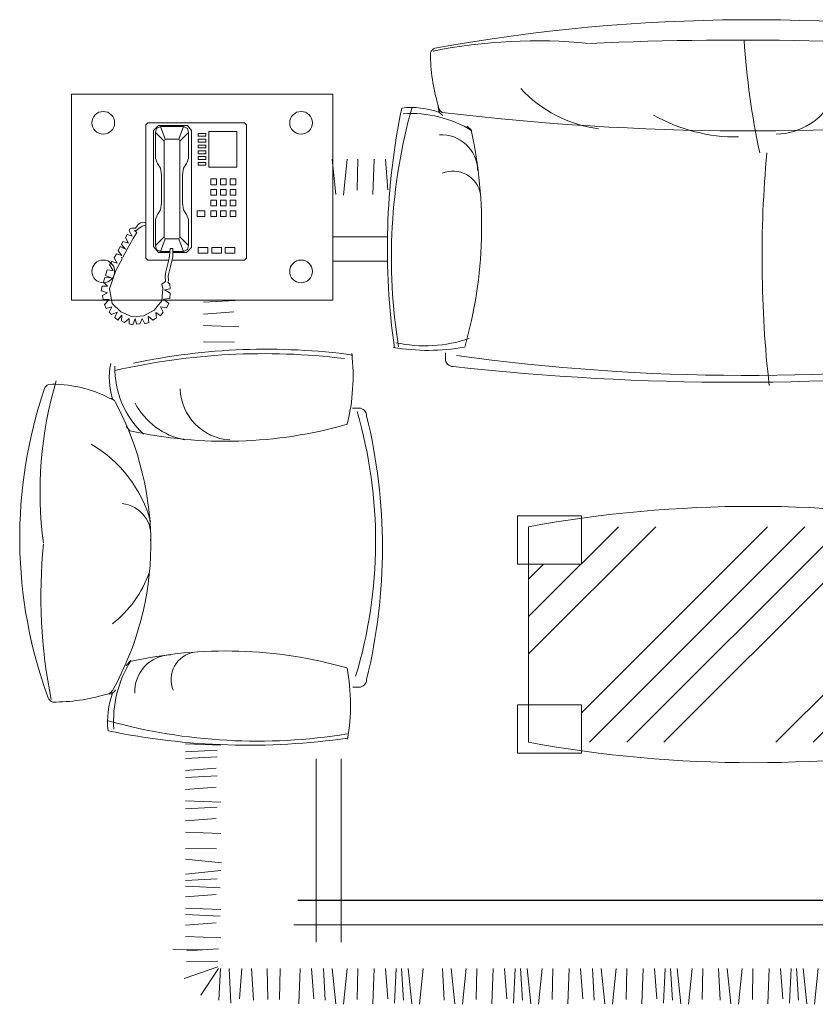
# Model space of a CAD drawing. Units: inches. Extents: x 1961 to 3038, y 800 to 1438.
# Tile 8 of 13: x 2866 to 2920, y 1028 to 1096. Entities that reach past the tile are written whole.
import ezdxf

# ---------------------------------------------------------------- set-up
doc = ezdxf.new("R2010")
doc.units = ezdxf.units.IN
doc.layers.add('A-FURN', color=8, linetype='Continuous', lineweight=18)

# ---------------------------------------------------------------- blocks, each defined once
blk = doc.blocks.new('A$C28C76B35')
for p, q in [((1695.2, 4127.1, -618.7), (2191.4, 4127.1, -618.7)), ((1695.2, 3498.2, -618.7), (1695.2, 4127.1, -618.7)), ((2191.4, 4127.1, -618.7), (2191.4, 3498.2, -618.7)), ((1713.2, 4040.6, -1415), (1717.4, 4055.2, -1415)), ((1717.2, 4055.4, 1292.3), (1729.2, 4053, 1292.3)), ((1660.8, 4030.7, -1415), (1666.5, 4036.8, -1415)), ((1666.5, 4017.5, -1415), (1660.8, 4030.7, -1415)), ((1666.5, 4036.8, -1415), (1679.2, 4030.2, -1415)), ((1675, 4043.9, -1415), (1684.4, 4047.6, -1415)), ((1679.2, 4030.2, -1415), (1675, 4043.9, -1415)), ((1684.4, 4047.6, -1415), (1697.1, 4036.3, -1415)), ((1722.6, 4035.9, -1415), (1687.2, 4029.3, -1415)), ((1696.5, 4050.9, 1292.3), (1706.1, 4052.8, 1292.3)), ((1697.1, 4036.3, -1415), (1696.7, 4050.9, -1415)), ((1706.1, 4052.8, -1415), (1713.2, 4040.6, -1415)), ((1766.9, 4020.3, -1415), (1722.6, 4035.9, -1415)), ((1729.2, 4052.8, -1415), (1729.2, 4040.1, -1415)), ((1729.2, 4040.1, -1415), (1738.6, 4050, -1415)), ((1738.4, 4050.1, 1292.3), (1749.4, 4046.8, 1292.3)), ((1749.5, 4046.7, -1415), (1749, 4031.6, -1415)), ((1749, 4031.6, -1415), (1754.2, 4045.3, -1415)), ((1754.2, 4045.3, -1415), (1768.3, 4041, -1415)), ((1768.3, 4041, -1415), (1766.9, 4026.9, -1415)), ((1766.9, 4026.9, -1415), (1780.6, 4035.4, -1415)), ((1780.6, 4035.4, -1415), (1788.2, 4030.2, -1415)), ((1788.2, 4030.2, -1415), (1784.4, 4017, -1415)), ((1641.5, 3999.6, -1415), (1645.3, 4007.1, -1415)), ((1645.3, 4007.1, -1415), (1659.4, 4005.7, -1415)), ((1647.2, 4015.6, -1415), (1653.8, 4023.1, -1415)), ((1659.4, 4005.7, -1415), (1647.2, 4015.6, -1415)), ((1653.8, 4023.1, -1415), (1666.5, 4017.5, -1415)), ((1667, 4008.5, -1415), (1655.2, 3981.2, -1415)), ((1687.2, 4029.3, -1415), (1667, 4008.5, -1415)), ((1794.3, 4005.2, -1415), (1766.9, 4020.3, -1415)), ((1784.4, 4017, -1415), (1797.1, 4024.1, -1415)), ((1798.1, 4006.6, -1415), (1794.3, 4005.2, -1415)), ((1797.1, 4024.1, -1415), (1807, 4018.9, -1415)), ((1799, 4003.3, -1415), (1798.1, 4006.6, -1415)), ((1807, 4018.9, -1415), (1802.8, 4006.2, -1415)), ((1802.8, 4006.2, -1415), (1813.6, 4014.7, -1415)), ((1813.6, 4014.7, -1415), (1824, 4009.9, -1415)), ((1824, 4009.9, -1415), (1818.3, 3997.2, -1415)), ((1818.3, 3997.2, -1415), (1829.2, 4007.1, -1415)), ((1829.2, 4007.1, -1415), (1836.7, 4003.3, -1415)), ((1635.8, 3979.3, -1415), (1638.2, 3988.3, -1415)), ((1638.2, 3988.3, -1415), (1650.9, 3988.7, -1415)), ((1650.9, 3988.7, -1415), (1641.5, 3999.6, -1415)), ((1818.3, 3993.5, -1415), (1799, 4003.3, -1415)), ((1843.8, 3978.4, -1415), (1818.3, 3993.5, -1415)), ((1836.7, 4003.3, -1415), (1832.5, 3989.7, -1415)), ((1832.5, 3989.7, -1415), (1846.2, 3997.2, -1415)), ((1846.2, 3997.2, -1415), (1853.2, 3993.5, -1415)), ((1853.2, 3993.5, -1415), (1849.5, 3981.2, -1415)), ((1849.5, 3981.2, -1415), (1861.7, 3988.7, -1415)), ((1861.7, 3988.7, -1415), (1866.9, 3986.9, -1415)), ((1866.9, 3986.9, -1415), (1868.3, 3981.7, -1415)), ((1650.9, 3974.1, -1415), (1635.8, 3979.3, -1415)), ((1637.3, 3970.8, -1415), (1650.9, 3974.1, -1415)), ((1638.2, 3962.8, -1415), (1637.3, 3970.8, -1415)), ((1650.9, 3957.2, -1415), (1638.2, 3962.8, -1415)), ((1655.2, 3981.2, -1415), (1657.5, 3952.9, -1415)), ((1857.9, 3969.9, -1415), (1843.8, 3978.4, -1415)), ((1862.7, 3975.5, -1415), (1857.9, 3969.9, -1415)), ((1862.7, 3970.8, -1415), (1862.7, 3975.5, -1415)), ((1865.5, 3968, -1415), (1862.7, 3970.8, -1415)), ((1869.7, 3961.9, -1415), (1865.5, 3968, -1415)), ((1868.3, 3981.7, -1415), (1868.8, 3973.2, -1415)), ((1868.8, 3973.2, -1415), (1877.7, 3966.6, -1415)), ((1873.5, 3956.7, -1415), (1869.7, 3961.9, -1415)), ((1877.7, 3966.6, -1415), (1881, 3960.9, -1415)), ((1881, 3960.9, -1415), (1882.4, 3948.1, -1415)), ((1638.2, 3951, -1415), (1650.9, 3957.2, -1415)), ((1641, 3941.1, -1415), (1638.2, 3951, -1415)), ((1656.6, 3942.6, -1415), (1641, 3941.1, -1415)), ((1647.2, 3931.2, -1415), (1656.6, 3942.6, -1415)), ((1657.5, 3952.9, -1415), (1670.7, 3927.9, -1415)), ((1796.3, 3948.1, -1415), (1791.6, 3943.4, -1415)), ((1791.6, 3943.4, -1415), (1791.6, 3893.2, -1415)), ((2117.6, 3948.1, -1415), (1796.3, 3948.1, -1415)), ((1875.4, 3948.1, -1415), (1873.5, 3956.7, -1415)), ((2122.3, 3943.4, -1415), (2117.6, 3948.1, -1415)), ((2122.3, 3710.5, -1415), (2122.3, 3943.4, -1415)), ((1652.8, 3922.3, -1415), (1647.2, 3931.2, -1415)), ((1665.6, 3924.2, -1415), (1652.8, 3922.3, -1415)), ((1657.5, 3913.3, -1415), (1665.6, 3924.2, -1415)), ((1666, 3906.3, -1415), (1657.5, 3913.3, -1415)), ((1679.2, 3912.9, -1415), (1666, 3906.3, -1415)), ((1670.7, 3927.9, -1415), (1693.4, 3910, -1415)), ((1676.4, 3898.7, -1415), (1679.2, 3912.9, -1415)), ((1824.2, 3929.4, -1415), (1810.2, 3917.8, -1415)), ((1810.2, 3917.8, -1415), (1810.2, 3890.5, -1415)), ((1812.6, 3913.1, -1415), (1817.2, 3922.4, -1415)), ((1812.6, 3890.3, -1415), (1812.6, 3913.1, -1415)), ((1842.8, 3901.5, -1415), (1812.6, 3913.1, -1415)), ((1817.2, 3922.4, -1415), (1826.5, 3924.8, -1415)), ((2103.6, 3929.4, -1415), (1824.2, 3929.4, -1415)), ((1826.5, 3924.8, -1415), (1889.4, 3924.8, -1415)), ((1826.5, 3924.8, -1415), (1847.5, 3903.8, -1415)), ((1889.4, 3924.8, -1415), (1901.1, 3920.1, -1415)), ((1901.1, 3920.1, -1415), (1912.7, 3913.1, -1415)), ((1912.7, 3913.1, -1415), (1929, 3910.8, -1415)), ((2012.8, 3913.1, -1415), (1996.5, 3910.8, -1415)), ((2024.5, 3920.1, -1415), (2012.8, 3913.1, -1415)), ((2036.1, 3924.8, -1415), (2024.5, 3920.1, -1415)), ((2099, 3924.8, -1415), (2036.1, 3924.8, -1415)), ((2099, 3924.8, -1415), (2078, 3903.8, -1415)), ((2082.7, 3901.5, -1415), (2112.9, 3913.1, -1415)), ((2108.3, 3922.4, -1415), (2099, 3924.8, -1415)), ((2115.3, 3917.8, -1415), (2103.6, 3929.4, -1415)), ((2112.9, 3913.1, -1415), (2108.3, 3922.4, -1415)), ((2112.9, 3857.2, -1415), (2112.9, 3913.1, -1415)), ((2115.3, 3847.9, -1415), (2115.3, 3917.8, -1415)), ((1687.2, 3892.6, -1415), (1676.4, 3898.7, -1415)), ((1697.6, 3905.8, -1415), (1687.2, 3892.6, -1415)), ((1693.4, 3910, -1415), (1723.1, 3907.7, -1415)), ((1699, 3890.7, -1415), (1697.6, 3905.8, -1415)), ((1711.8, 3889.8, -1415), (1699, 3890.7, -1415)), ((1719.8, 3903, -1415), (1711.8, 3889.8, -1415)), ((1722.1, 3889.3, -1415), (1719.8, 3903, -1415)), ((1733.5, 3890.2, -1415), (1722.1, 3889.3, -1415)), ((1723.1, 3907.7, -1415), (1733.9, 3909.6, -1415)), ((1738.6, 3895.4, -1415), (1733.5, 3890.2, -1415)), ((1733.9, 3909.6, -1415), (1740.1, 3901.1, -1415)), ((1741.5, 3894, -1415), (1738.6, 3895.4, -1415)), ((1740.1, 3901.1, -1415), (1752.3, 3901.6, -1415)), ((1753.7, 3894.5, -1415), (1741.5, 3894, -1415)), ((1752.3, 3901.6, -1415), (1763.6, 3900.1, -1415)), ((1775.9, 3888.8, -1415), (1753.7, 3894.5, -1415)), ((1763.6, 3900.1, -1415), (1785.8, 3894.5, -1415)), ((1799.5, 3883.2, -1415), (1775.9, 3888.8, -1415)), ((1785.8, 3894.5, -1415), (1800.9, 3891.2, -1415)), ((1800.9, 3891.2, -1415), (1819.6, 3889.8, -1415)), ((1819.6, 3889.8, -1415), (1819.6, 3882.9, -1415)), ((1847.5, 3903.8, -1415), (1842.8, 3901.5, -1415)), ((1842.8, 3901.5, -1415), (1842.8, 3868.9, -1415)), ((1973.2, 3903.8, -1415), (1847.5, 3903.8, -1415)), ((1929, 3910.8, -1415), (1973.2, 3910.8, -1415)), ((1996.5, 3910.8, -1415), (1973.2, 3910.8, -1415)), ((1973.2, 3903.8, -1415), (2078, 3903.8, -1415)), ((2078, 3903.8, -1415), (2082.7, 3901.5, -1415)), ((2082.7, 3901.5, -1415), (2082.7, 3868.9, -1415)), ((131, 3801, -715.1), (132.6, 3883.3, -715.1)), ((1791.6, 3885.1, -1415), (1791.6, 3710.5, -1415)), ((1819.6, 3882.9, -1415), (1799.5, 3883.2, -1415)), ((1810.2, 3883, -1415), (1810.2, 3850.3, -1415)), ((1812.6, 3857.2, -1415), (1812.6, 3883, -1415)), ((1842.8, 3868.9, -1415), (1812.6, 3857.2, -1415)), ((1826.5, 3845.6, -1415), (1847.5, 3866.6, -1415)), ((1847.5, 3866.6, -1415), (1842.8, 3868.9, -1415)), ((1973.2, 3866.6, -1415), (1847.5, 3866.6, -1415)), ((1973.2, 3866.6, -1415), (2078, 3866.6, -1415)), ((2078, 3866.6, -1415), (2082.7, 3868.9, -1415)), ((2099, 3845.6, -1415), (2078, 3866.6, -1415)), ((2082.7, 3868.9, -1415), (2112.9, 3857.2, -1415)), ((89.9, 3775.3, -715.1), (61.8, 3856, -715.1)), ((103.7, 3775.7, -715.1), (102.2, 3850.5, -715.1)), ((133.3, 3773.3, -715.1), (129, 3849.6, -715.1)), ((162.9, 3852.6, -715.1), (160, 3767.7, -715.1)), ((190.2, 3852.6, -715.1), (196, 3779.2, -715.1)), ((216.2, 3852.6, -715.1), (211.9, 3769.2, -715.1)), ((231.4, 3852.6, -715.1), (228.6, 3767.7, -715.1)), ((258.8, 3852.6, -715.1), (264.6, 3779.2, -715.1)), ((284.7, 3852.6, -715.1), (280.4, 3769.2, -715.1)), ((297.7, 3852.6, -715.1), (302, 3776.4, -715.1)), ((313.5, 3852.6, -715.1), (322.2, 3767.7, -715.1)), ((349.5, 3852.6, -715.1), (340.9, 3766.3, -715.1)), ((375.4, 3852.6, -715.1), (374, 3777.8, -715.1)), ((414.3, 3852.6, -715.1), (411.5, 3767.7, -715.1)), ((441.7, 3852.6, -715.1), (447.5, 3779.2, -715.1)), ((470.4, 3852.6, -715.1), (474.7, 3776.4, -715.1)), ((489.7, 3852.6, -715.1), (486.9, 3767.7, -715.1)), ((517.1, 3852.6, -715.1), (522.9, 3779.2, -715.1)), ((545.8, 3852.6, -715.1), (550.1, 3776.4, -715.1)), ((562.8, 3852.6, -715.1), (568.6, 3779.2, -715.1)), ((591.5, 3852.6, -715.1), (595.8, 3776.4, -715.1)), ((607.5, 3852.6, -715.1), (611.8, 3776.4, -715.1)), ((626.8, 3852.6, -715.1), (623.9, 3767.7, -715.1)), ((1810.2, 3850.3, -1415), (1821.9, 3838.6, -1415)), ((1812.6, 3857.2, -1415), (1817.2, 3847.9, -1415)), ((1817.2, 3847.9, -1415), (1826.5, 3845.6, -1415)), ((1826.5, 3845.6, -1415), (1889.4, 3845.6, -1415)), ((1889.4, 3845.6, -1415), (1901.1, 3850.3, -1415)), ((1901.1, 3850.3, -1415), (1912.7, 3857.2, -1415)), ((1912.7, 3857.2, -1415), (1929, 3859.6, -1415)), ((1929, 3859.6, -1415), (1973.2, 3859.6, -1415)), ((1996.5, 3859.6, -1415), (1973.2, 3859.6, -1415)), ((2012.8, 3857.2, -1415), (1996.5, 3859.6, -1415)), ((2024.5, 3850.3, -1415), (2012.8, 3857.2, -1415)), ((2036.1, 3845.6, -1415), (2024.5, 3850.3, -1415)), ((2099, 3845.6, -1415), (2036.1, 3845.6, -1415)), ((2108.3, 3847.9, -1415), (2099, 3845.6, -1415)), ((2103.6, 3838.6, -1415), (2115.3, 3847.9, -1415)), ((2112.9, 3857.2, -1415), (2108.3, 3847.9, -1415)), ((1807.9, 3822.3, -1415), (1821.9, 3822.3, -1415)), ((1807.9, 3799, -1415), (1807.9, 3822.3, -1415)), ((1821.9, 3838.6, -1415), (2103.6, 3838.6, -1415)), ((1821.9, 3822.3, -1415), (1821.9, 3799, -1415)), ((1910.4, 3824.6, -1415), (1896.4, 3824.6, -1415)), ((1896.4, 3824.6, -1415), (1896.4, 3806, -1415)), ((1910.4, 3806, -1415), (1910.4, 3824.6, -1415)), ((2019.8, 3822.3, -1415), (2026.8, 3822.3, -1415)), ((2019.8, 3803.7, -1415), (2019.8, 3822.3, -1415)), ((2026.8, 3822.3, -1415), (2026.8, 3803.7, -1415)), ((2033.8, 3822.3, -1415), (2040.8, 3822.3, -1415)), ((2033.8, 3803.7, -1415), (2033.8, 3822.3, -1415)), ((2040.8, 3822.3, -1415), (2040.8, 3803.7, -1415)), ((2047.7, 3822.3, -1415), (2054.7, 3822.3, -1415)), ((2047.7, 3803.7, -1415), (2047.7, 3822.3, -1415)), ((2054.7, 3822.3, -1415), (2054.7, 3803.7, -1415)), ((2061.7, 3822.3, -1415), (2068.7, 3822.3, -1415)), ((2061.7, 3803.7, -1415), (2061.7, 3822.3, -1415)), ((2068.7, 3822.3, -1415), (2068.7, 3803.7, -1415)), ((2075.7, 3822.3, -1415), (2082.7, 3822.3, -1415)), ((2075.7, 3803.7, -1415), (2075.7, 3822.3, -1415)), ((2082.7, 3822.3, -1415), (2082.7, 3803.7, -1415)), ((2089.7, 3822.3, -1415), (2096.6, 3822.3, -1415)), ((2089.7, 3803.7, -1415), (2089.7, 3822.3, -1415)), ((2096.6, 3822.3, -1415), (2096.6, 3803.7, -1415)), ((85.9, 3773.7, -715.1), (22.2, 3815.6, -715.1)), ((1595.1, 3809.5, -715.1), (1593.7, 3734.7, -715.1)), ((1634, 3809.5, -715.1), (1631.1, 3724.6, -715.1)), ((1661.4, 3809.5, -715.1), (1667.1, 3736.1, -715.1)), ((1690.1, 3809.5, -715.1), (1694.4, 3733.2, -715.1)), ((1821.9, 3799, -1415), (1807.9, 3799, -1415)), ((1896.4, 3806, -1415), (1910.4, 3806, -1415)), ((2101.3, 3796.7, -1415), (2015.1, 3796.7, -1415)), ((2015.1, 3796.7, -1415), (2015.1, 3729.2, -1415)), ((2026.8, 3803.7, -1415), (2019.8, 3803.7, -1415)), ((2040.8, 3803.7, -1415), (2033.8, 3803.7, -1415)), ((2054.7, 3803.7, -1415), (2047.7, 3803.7, -1415)), ((2068.7, 3803.7, -1415), (2061.7, 3803.7, -1415)), ((2082.7, 3803.7, -1415), (2075.7, 3803.7, -1415)), ((2096.6, 3803.7, -1415), (2089.7, 3803.7, -1415)), ((2101.3, 3729.2, -1415), (2101.3, 3796.7, -1415)), ((86.3, 3768.2, -715.1), (10.1, 3772.5, -715.1)), ((1807.9, 3789.7, -1415), (1821.9, 3789.7, -1415)), ((1807.9, 3766.4, -1415), (1807.9, 3789.7, -1415)), ((1821.9, 3789.7, -1415), (1821.9, 3766.4, -1415)), ((1910.4, 3792, -1415), (1896.4, 3792, -1415)), ((1896.4, 3792, -1415), (1896.4, 3778.1, -1415)), ((1896.4, 3778.1, -1415), (1910.4, 3778.1, -1415)), ((1910.4, 3778.1, -1415), (1910.4, 3792, -1415)), ((1936, 3792, -1415), (1922, 3792, -1415)), ((1922, 3792, -1415), (1922, 3778.1, -1415)), ((1922, 3778.1, -1415), (1936, 3778.1, -1415)), ((1936, 3778.1, -1415), (1936, 3792, -1415)), ((1961.6, 3792, -1415), (1947.6, 3792, -1415)), ((1947.6, 3792, -1415), (1947.6, 3778.1, -1415)), ((1947.6, 3778.1, -1415), (1961.6, 3778.1, -1415)), ((1961.6, 3778.1, -1415), (1961.6, 3792, -1415)), ((1987.2, 3792, -1415), (1973.2, 3792, -1415)), ((1973.2, 3792, -1415), (1973.2, 3778.1, -1415)), ((1973.2, 3778.1, -1415), (1987.2, 3778.1, -1415)), ((1987.2, 3778.1, -1415), (1987.2, 3792, -1415)), ((86.3, 3747.6, -715.1), (2.9, 3743.3, -715.1)), ((1821.9, 3766.4, -1415), (1807.9, 3766.4, -1415)), ((1807.9, 3757.1, -1415), (1821.9, 3757.1, -1415)), ((1807.9, 3733.8, -1415), (1807.9, 3757.1, -1415)), ((1821.9, 3757.1, -1415), (1821.9, 3733.8, -1415)), ((1896.4, 3768.8, -1415), (1896.4, 3754.8, -1415)), ((1910.4, 3768.8, -1415), (1896.4, 3768.8, -1415)), ((1896.4, 3754.8, -1415), (1910.4, 3754.8, -1415)), ((1910.4, 3745.5, -1415), (1896.4, 3745.5, -1415)), ((1896.4, 3745.5, -1415), (1896.4, 3731.5, -1415)), ((1910.4, 3754.8, -1415), (1910.4, 3768.8, -1415)), ((1910.4, 3731.5, -1415), (1910.4, 3745.5, -1415)), ((1922, 3768.8, -1415), (1922, 3754.8, -1415)), ((1936, 3768.8, -1415), (1922, 3768.8, -1415)), ((1922, 3754.8, -1415), (1936, 3754.8, -1415)), ((1936, 3745.5, -1415), (1922, 3745.5, -1415)), ((1922, 3745.5, -1415), (1922, 3731.5, -1415)), ((1936, 3754.8, -1415), (1936, 3768.8, -1415)), ((1936, 3731.5, -1415), (1936, 3745.5, -1415)), ((1961.6, 3768.8, -1415), (1947.6, 3768.8, -1415)), ((1947.6, 3768.8, -1415), (1947.6, 3754.8, -1415)), ((1947.6, 3754.8, -1415), (1961.6, 3754.8, -1415)), ((1961.6, 3745.5, -1415), (1947.6, 3745.5, -1415)), ((1947.6, 3745.5, -1415), (1947.6, 3731.5, -1415)), ((1961.6, 3754.8, -1415), (1961.6, 3768.8, -1415)), ((1961.6, 3731.5, -1415), (1961.6, 3745.5, -1415)), ((1973.2, 3768.8, -1415), (1973.2, 3754.8, -1415)), ((1987.2, 3768.8, -1415), (1973.2, 3768.8, -1415)), ((1973.2, 3754.8, -1415), (1987.2, 3754.8, -1415)), ((1987.2, 3745.5, -1415), (1973.2, 3745.5, -1415)), ((1973.2, 3745.5, -1415), (1973.2, 3731.5, -1415)), ((1987.2, 3754.8, -1415), (1987.2, 3768.8, -1415)), ((1987.2, 3731.5, -1415), (1987.2, 3745.5, -1415)), ((86.3, 3717.2, -715.1), (13, 3722.9, -715.1)), ((1821.9, 3733.8, -1415), (1807.9, 3733.8, -1415)), ((1896.4, 3731.5, -1415), (1910.4, 3731.5, -1415)), ((1922, 3731.5, -1415), (1936, 3731.5, -1415)), ((1947.6, 3731.5, -1415), (1961.6, 3731.5, -1415)), ((1973.2, 3731.5, -1415), (1987.2, 3731.5, -1415)), ((2015.1, 3729.2, -1415), (2101.3, 3729.2, -1415)), ((1791.6, 3710.5, -1415), (1796.3, 3705.9, -1415)), ((1796.3, 3705.9, -1415), (2117.6, 3705.9, -1415)), ((2117.6, 3705.9, -1415), (2122.3, 3710.5, -1415)), ((86.3, 3693.6, -715.1), (10.1, 3689.3, -715.1)), ((86.3, 3656.5, -715.1), (11.5, 3655, -715.1)), ((86.3, 3625, -715.1), (11.5, 3626.4, -715.1)), ((86.3, 3577, -715.1), (1.4, 3579.9, -715.1)), ((86.3, 3549.6, -715.1), (13, 3543.9, -715.1)), ((149.4, 3538.6), (591.1, 3538.6)), ((86.3, 3520.9, -715.1), (10.1, 3516.6, -715.1)), ((86.3, 3499.8, -715.1), (1.4, 3491.1, -715.1)), ((2191.4, 3498.2, -618.7), (1695.2, 3498.2, -618.7)), ((1788.8, 3366.7, -715.1), (1788.8, 3498.2, -715.1)), ((1847.7, 3366.8, -715.1), (1847.7, 3498.2, -715.1)), ((2034.4, 3499.8, -715.1), (1949.5, 3491.1, -715.1)), ((86.3, 3463.8, -715.1), (0, 3472.4, -715.1)), ((149.4, 3478.3), (591.1, 3478.3)), ((2034.4, 3463.8, -715.1), (1948.1, 3472.4, -715.1)), ((86.3, 3437.9, -715.1), (11.5, 3439.3, -715.1)), ((763.3, 3449.9, -2545.7), (763.3, 3435.6, -2545.7)), ((1435.3, 3450.9, -2545.7), (1435.3, 3435.6, -2545.7)), ((2034.4, 3437.9, -715.1), (1959.6, 3439.3, -715.1)), ((86.3, 3399, -715.1), (1.4, 3401.8, -715.1)), ((2034.4, 3399, -715.1), (1949.5, 3401.8, -715.1)), ((86.3, 3371.6, -715.1), (13, 3365.8, -715.1)), ((2034.4, 3371.6, -715.1), (1961, 3365.8, -715.1)), ((86.3, 3345.7, -715.1), (2.9, 3350, -715.1)), ((86.3, 3332.7, -715.1), (10.1, 3328.4, -715.1)), ((86.3, 3316.9, -715.1), (1.4, 3308.2, -715.1)), ((86.3, 3280.9, -715.1), (0, 3289.5, -715.1)), ((86.3, 3234.6, -715.1), (10.1, 3230.3, -715.1)), ((1568.5, 3227.4, -2545.7), (1554.2, 3227.4, -2545.7)), ((86.3, 3213.4, -715.1), (1.4, 3204.8, -715.1)), ((86.3, 3177.4, -715.1), (0, 3186.1, -715.1)), ((86.3, 3151.5, -715.1), (11.5, 3152.9, -715.1)), ((86.3, 3112.6, -715.1), (1.4, 3115.5, -715.1)), ((86.3, 3085.3, -715.1), (13, 3079.5, -715.1)), ((86.3, 3059.3, -715.1), (2.9, 3063.7, -715.1)), ((86.3, 3046.4, -715.1), (10.1, 3042, -715.1)), ((86.3, 3030.5, -715.1), (1.4, 3021.9, -715.1)), ((1149.7, 3027.1), (630.8, 3027.1)), ((843.8, 3027.1), (1149.7, 2721.2)), ((933.6, 3027.1), (1059.7, 2901.1)), ((1023.4, 3027.1), (1059.7, 2990.9)), ((86.3, 2994.5, -715.1), (0, 3003.2, -715.1)), ((86.3, 2968.6, -715.1), (11.5, 2970, -715.1)), ((86.3, 2929.7, -715.1), (1.4, 2932.6, -715.1)), ((86.3, 2902.4, -715.1), (13, 2896.6, -715.1)), ((701.6, 2899.9), (1149.7, 2451.8)), ((1060.8, 2899.9), (1149.7, 2811)), ((86.3, 2873.7, -715.1), (10.1, 2869.3, -715.1)), ((630.8, 2880.9), (1149.7, 2362)), ((86.3, 2852.5, -715.1), (1.4, 2843.9, -715.1)), ((86.3, 2816.5, -715.1), (0, 2825.2, -715.1)), ((86.3, 2790.6, -715.1), (11.5, 2792, -715.1)), ((630.8, 2791.1), (1149.7, 2272.2)), ((86.3, 2751.7, -715.1), (1.4, 2754.6, -715.1)), ((86.3, 2698.4, -715.1), (2.9, 2702.7, -715.1)), ((86.3, 2724.3, -715.1), (13, 2718.6, -715.1)), ((86.3, 2685.5, -715.1), (10.1, 2681.1, -715.1)), ((630.8, 2701.3), (1149.7, 2182.4)), ((86.3, 2669.6, -715.1), (1.4, 2661, -715.1)), ((86.3, 2633.6, -715.1), (0, 2642.3, -715.1)), ((86.3, 2607.7, -715.1), (11.5, 2609.1, -715.1)), ((86.3, 2570.3, -715.1), (10.1, 2566, -715.1)), ((86.3, 2549.1, -715.1), (1.4, 2540.5, -715.1)), ((86.3, 2513.1, -715.1), (0, 2521.8, -715.1)), ((86.3, 2487.2, -715.1), (11.5, 2488.6, -715.1)), ((86.3, 2448.3, -715.1), (1.4, 2451.2, -715.1)), ((86.3, 2421, -715.1), (13, 2415.2, -715.1)), ((630.8, 2431.9), (1059.7, 2003)), ((86.3, 2395, -715.1), (2.9, 2399.4, -715.1)), ((86.3, 2382.1, -715.1), (10.1, 2377.8, -715.1)), ((86.3, 2366.2, -715.1), (1.4, 2357.6, -715.1)), ((86.3, 2330.2, -715.1), (0, 2338.9, -715.1)), ((630.8, 2342.1), (1027.2, 1945.7))]:
    blk.add_line(p, q)
at = {"const_width": 2.63, "elevation": -715.1}
for points in [[(191.4, 983.4), (191.4, 3592.6)], [(250.4, 983.4), (250.4, 3582.8)]]:
    blk.add_lwpolyline(points, dxfattribs=at)
for points in [[(604.3, 3053.6), (604.3, 2899.9), (720.8, 2899.9), (720.8, 3053.6)], [(1176.1, 3053.6), (1176.1, 2899.9), (1059.7, 2899.9), (1059.7, 3053.6)]]:
    blk.add_lwpolyline(points, close=True)
for centre in [(1764.5, 4050.6, -691), (2122.2, 4050.6, -691), (1764.5, 3574.7, -691), (2122.2, 3574.7, -691)]:
    blk.add_circle(centre, 27.3)
for centre, radius, start, end in [((1122.4, 3139.3, -2545.7), 1112.4, 71.1157, 110.2204), ((982.3, 2946.4, -2545.7), 1254.5, 84.253, 101.4358), ((1233, 3266.2, -2545.7), 936.6, 73.3816, 97.55), ((745.4, 4166, -2545.7), 18.8, 113.3322, 161.3637), ((1166.3, 4171, -2545.7), 438.7, 179.879, 196.6328), ((745.3, 4165.9, -2545.7), 18.8, 114.0758, 156.3315), ((1205.3, 4170.7, -2545.7), 287.4, 332.1884, 2.3768), ((1475.5, 4174.4, -2545.7), 18.8, 25.7033, 68.2144), ((1081.1, 4236, -2545.7), 309.7, 284.9836, 329.7062), ((2293.5, 3700.5, -2545.7), 1669.8, 168.3019, 188.2166), ((1979.1, 3679.3, -2545.7), 1345.6, 164.4911, 189.2138), ((681.1, 3841.3, -2545.7), 199.1, 69.9615, 96.5551), ((764.7, 4044.8, -2545.7), 18.8, 177.437, 237.6208), ((764.7, 4044.8, -2545.7), 18.8, 178.0201, 240.7828), ((765.3, 4038.1, -2545.7), 18.8, 184.7243, 243.4779), ((1440.8, 4038.1, -2545.7), 18.8, 296.5221, 355.2757), ((1508.7, 3860.6, -2545.7), 175.5, 78.8784, 107.2062), ((680.4, 3745.3, -2545.7), 280.7, 58.4292, 93.73), ((1108.8, 4660.1, -2545.7), 723.8, 240.7828, 298.0488), ((1129.3, 4195.2, -2545.7), 270.6, 217.955, 250.4125), ((1531.6, 3804.2, -2545.7), 218.5, 88.8733, 136.7696), ((-30.8, 3664.2, -2545.7), 1597.2, 353.0352, 12.9689), ((-213.3, 3755.4, -2545.7), 1063.9, 344.0709, 12.558), ((705.6, 3858.8, -2545.7), 175.1, 46.9453, 51.4779), ((1128.9, 4012.9, -2545.7), 77, 261.0221, 354.0715), ((2419.4, 3755.4, -2545.7), 1063.9, 167.442, 195.9291), ((1500.5, 3858.8, -2545.7), 175.1, 128.5221, 133.0547), ((754.2, 3887.7, -2545.7), 86.8, 1.0101, 93.44), ((1528.8, 3821.3, -2545.7), 173.3, 118.0169, 168.7258), ((36.7, 3657.4, -2379.3), 1540.4, 352.251, 12.0202), ((781.6, 3820.4, -2545.7), 67.1, 9.3795, 112.5496), ((1484.9, 3739.1, -2545.7), 126.3, 91.587, 176.7541), ((721.7, 3942.2, -2545.7), 486.5, 260.0867, 280.4034), ((1512.5, 3932.4, -2545.7), 482.9, 256.0947, 276.4886), ((1114.1, 4512.2, -2545.7), 1117, 253.1262, 286.2615), ((782.1, 3435.6, -2545.7), 18.8, 180, 270), ((1099.3, 4723.9, -2545.7), 1345, 256.3605, 283.6395), ((1416.5, 3435.6, -2545.7), 18.8, 270, 0), ((1819.1, 1697.2, -2545.7), 1669.8, 78.3019, 98.2166), ((2060.8, 3269, -2545.7), 486.5, 170.0867, 190.4034), ((1797.9, 2011.6, -2545.7), 1345.6, 74.4911, 99.2138), ((1916.8, 3276.6, -2545.7), 331.6, 167.8205, 198.7312), ((1863.9, 3310.3, -2545.7), 280.7, 328.4292, 3.73), ((1959.9, 3309.6, -2545.7), 199.1, 339.9615, 6.5551), ((2289.6, 2824.4, -2545.7), 438.7, 89.879, 106.6328), ((2284.6, 3245.3, -2545.7), 18.8, 23.3322, 71.3637), ((2284.5, 3245.4, -2545.7), 18.8, 24.0758, 66.3315), ((1065, 3008.4, -2545.7), 1254.5, 354.253, 11.4358), ((-1923.8, 2488.5, -2545.7), 4294.1, 350.4205, 10.2522), ((1554.2, 3208.6, -2545.7), 18.8, 90, 180), ((1939, 3209.1, -2545.7), 67.1, 279.3795, 22.5496), ((2006.3, 3236.5, -2545.7), 86.8, 271.0101, 3.44), ((8358.1, 2490.4, -2545.7), 6255.6, 173.16241, 186.27001), ((2156.7, 3225.4, -2545.7), 18.8, 94.7243, 153.4779), ((2163.4, 3226, -2545.7), 18.8, 88.0201, 150.7828), ((2163.4, 3226, -2545.7), 18.8, 87.437, 147.6208), ((7689.8, 2524.2, -2545.7), 6192.4, 173.65504, 186.34496), ((6606.3, 2502.6, -2545.7), 5092.4, 172.1196, 187.596), ((1874, 4204, -2545.7), 1063.9, 254.0709, 282.558), ((1977.4, 3285.1, -2545.7), 175.1, 316.9453, 321.4779), ((2418.5, 2816.9, -2545.7), 313.5, 133.01, 172.2904), ((3583.6, 2486.4), 3001.9, 169.6234, 190.3766), ((-1803.1, 2486.4), 3001.9, 349.6234, 10.3766), ((-5321.3, 2528, -2545.7), 7642.7, 354.19861, 2.64527), ((2490.2, 2527.1, -2545.7), 402.2, 150.296, 180.7853), ((2449.4, 587.3, -2545.7), 1925.5, 93.8125, 101.9792), ((1797.7, -294.8, -2545.7), 2760.1, 84.7609, 96.4092), ((2254.5, 2435.4, -2545.7), 160, 181.4899, 243.2939)]:
    blk.add_arc(centre, radius, start, end)

msp = doc.modelspace()

# ---------------------------------------------------------------- block references
at = {"layer": 'A-FURN', "xscale": 0.0283328092017671, "yscale": 0.0283328092017671, "zscale": 0.0283328092017671, "rotation": 90}
msp.add_blockref('A$C28C76B35', (2986.6849, 1028.46179, 88.65501), dxfattribs=at)

doc.saveas('drawing.dxf')
